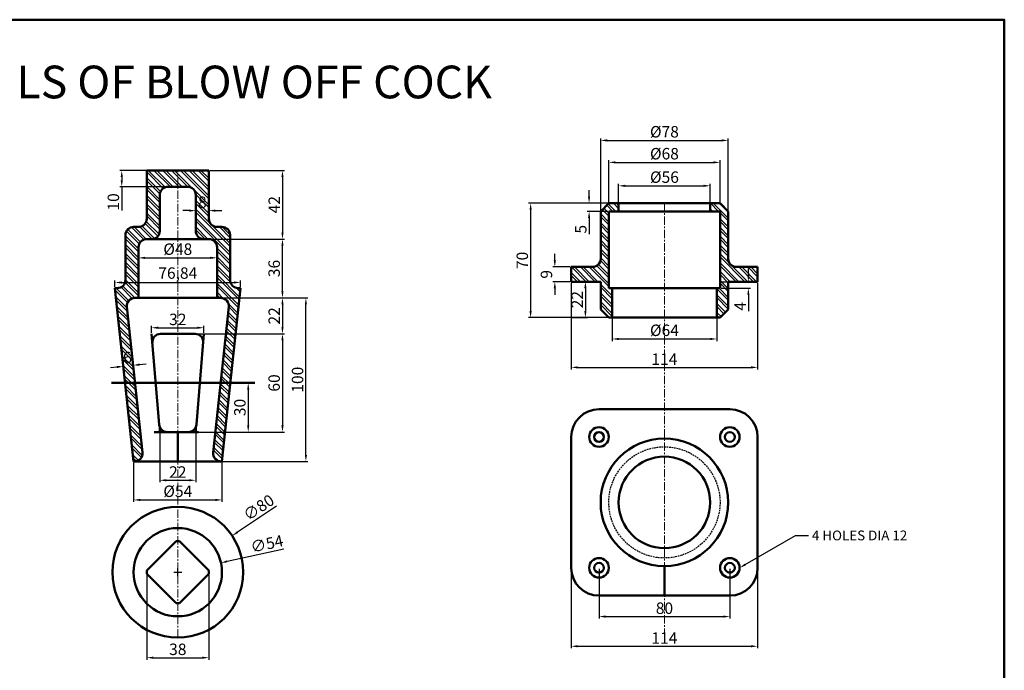
# Model space of a CAD drawing. Units: millimetres. Extents: x 49 to 1001, y -335 to 311.
# Tile 4 of 4: x 399 to 1001, y -87 to 311. Entities that reach past the tile are written whole.
import ezdxf
from ezdxf import colors
from ezdxf.entities.mleader import LeaderData, LeaderLine
from ezdxf.math import Vec2, Vec3

# ---------------------------------------------------------------- set-up
doc = ezdxf.new("R2010")
doc.units = ezdxf.units.MM
doc.header["$LTSCALE"] = 0.4
doc.linetypes.add('CENTER', pattern=[50.8, 31.75, -6.35, 6.35, -6.35])
doc.linetypes.add('HIDDEN', pattern=[9.525, 6.35, -3.175])
for name, color, linetype, lineweight in [('M-CNTR', 1, 'CENTER', 18), ('M-DIMS', 2, 'Continuous', 25), ('M-HATC', 8, 'Continuous', 18), ('M-HIDN', 6, 'HIDDEN', 25), ('M-OUTL', 7, 'Continuous', 50), ('M-TEXT', 3, 'Continuous', 25)]:
    doc.layers.add(name, color=color, linetype=linetype, lineweight=lineweight)
doc.styles.get("Standard").update_dxf_attribs({"font": 'arial.ttf'})
doc.dimstyles.new('ISO-25', dxfattribs={"dimtxt": 7, "dimasz": 4, "dimexe": 1.25, "dimexo": 0.625, "dimtad": 1, "dimtxsty": 'Standard', "dimcen": 2.5, "dimadec": 0, "dimazin": 0, "dimtfac": 1, "dimtofl": 0, "dimtmove": 0, "dimatfit": 3, "dimfxl": 1, "dimarcsym": 0})

# ---------------------------------------------------------------- blocks, each defined once
blk = doc.blocks.new('*D24')
at = {"layer": 'Defpoints', "color": 0, "ltscale": 0.4, "transparency": 16777216}
for p in [(495.83, 219.19), (461.55, 209.19), (495.83, 209.19)]:
    blk.add_point(p, dxfattribs=at)
at = {"layer": 'M-DIMS', "color": 0, "lineweight": -2, "ltscale": 0.4, "transparency": 16777216}
for p, q in [((495.21, 219.19), (460.3, 219.19)), ((461.55, 215.19), (461.55, 213.19)), ((495.21, 209.19), (460.3, 209.19)), ((461.55, 209.19), (461.55, 194.6))]:
    blk.add_line(p, q, dxfattribs=at)
at = {"layer": 'M-DIMS', "color": 0, "ltscale": 0.4, "transparency": 16777216}
for points in [[(460.89, 215.19), (462.22, 215.19), (461.55, 219.19)], [(460.89, 213.19), (462.22, 213.19), (461.55, 209.19)]]:
    blk.add_solid(points, dxfattribs=at)
at = {"layer": 'M-DIMS', "color": 0, "ltscale": 0.4, "transparency": 16777216, "insert": (457.35, 199.9), "char_height": 7, "attachment_point": 5, "rotation": 90}
blk.add_mtext('10', dxfattribs=at)
blk = doc.blocks.new('*D25')
at = {"layer": 'Defpoints', "color": 0, "ltscale": 0.4, "transparency": 16777216}
for p in [(514.83, 219.19), (495.83, 177.19), (559.86, 177.19)]:
    blk.add_point(p, dxfattribs=at)
at = {"layer": 'M-DIMS', "color": 0, "lineweight": -2, "ltscale": 0.4, "transparency": 16777216}
for p, q in [((515.46, 219.19), (561.11, 219.19)), ((559.86, 215.19), (559.86, 181.19)), ((496.46, 177.19), (561.11, 177.19))]:
    blk.add_line(p, q, dxfattribs=at)
at = {"layer": 'M-DIMS', "color": 0, "ltscale": 0.4, "transparency": 16777216}
for points in [[(559.19, 215.19), (560.52, 215.19), (559.86, 219.19)], [(559.19, 181.19), (560.52, 181.19), (559.86, 177.19)]]:
    blk.add_solid(points, dxfattribs=at)
at = {"layer": 'M-DIMS', "color": 0, "ltscale": 0.4, "transparency": 16777216, "insert": (555.72, 198.19), "char_height": 7, "attachment_point": 5, "rotation": 90}
blk.add_mtext('42', dxfattribs=at)
blk = doc.blocks.new('*D26')
at = {"layer": 'Defpoints', "color": 0, "ltscale": 0.4, "transparency": 16777216}
for p in [(506.83, 196.43), (514.83, 196.43), (514.83, 194.58)]:
    blk.add_point(p, dxfattribs=at)
at = {"layer": 'M-DIMS', "color": 0, "lineweight": -2, "ltscale": 0.4, "transparency": 16777216}
for p, q in [((502.83, 194.58), (498.83, 194.58)), ((506.83, 195.81), (506.83, 193.33)), ((514.83, 195.81), (514.83, 193.33)), ((518.83, 194.58), (522.83, 194.58))]:
    blk.add_line(p, q, dxfattribs=at)
at = {"layer": 'M-DIMS', "color": 0, "ltscale": 0.4, "transparency": 16777216}
for points in [[(502.83, 195.25), (502.83, 193.91), (506.83, 194.58)], [(518.83, 195.25), (518.83, 193.91), (514.83, 194.58)]]:
    blk.add_solid(points, dxfattribs=at)
at = {"layer": 'M-DIMS', "color": 0, "ltscale": 0.4, "transparency": 16777216, "insert": (510.83, 198.78), "char_height": 7, "attachment_point": 5}
blk.add_mtext('8', dxfattribs=at)
blk = doc.blocks.new('*D27')
at = {"layer": 'Defpoints', "color": 0, "ltscale": 0.4, "transparency": 16777216}
for p in [(468.83, 41.19), (522.83, 41.19), (522.83, 17.66)]:
    blk.add_point(p, dxfattribs=at)
at = {"layer": 'M-DIMS', "color": 0, "lineweight": -2, "ltscale": 0.4, "transparency": 16777216}
for p, q in [((468.83, 40.57), (468.83, 16.41)), ((522.83, 40.57), (522.83, 16.41)), ((472.83, 17.66), (518.83, 17.66))]:
    blk.add_line(p, q, dxfattribs=at)
at = {"layer": 'M-DIMS', "color": 0, "ltscale": 0.4, "transparency": 16777216}
for points in [[(472.83, 18.32), (472.83, 16.99), (468.83, 17.66)], [(518.83, 18.32), (518.83, 16.99), (522.83, 17.66)]]:
    blk.add_solid(points, dxfattribs=at)
at = {"layer": 'M-DIMS', "color": 0, "ltscale": 0.4, "transparency": 16777216, "insert": (495.83, 22.05), "char_height": 7, "attachment_point": 5}
blk.add_mtext('%%C54', dxfattribs=at)
blk = doc.blocks.new('*D28')
at = {"layer": 'Defpoints', "color": 0, "ltscale": 0.4, "transparency": 16777216}
for p in [(484.83, 59.19), (506.83, 59.19), (506.83, 29.68)]:
    blk.add_point(p, dxfattribs=at)
at = {"layer": 'M-DIMS', "color": 0, "lineweight": -2, "ltscale": 0.4, "transparency": 16777216}
for p, q in [((484.83, 58.57), (484.83, 28.43)), ((506.83, 58.57), (506.83, 28.43)), ((488.83, 29.68), (502.83, 29.68))]:
    blk.add_line(p, q, dxfattribs=at)
at = {"layer": 'M-DIMS', "color": 0, "ltscale": 0.4, "transparency": 16777216}
for points in [[(488.83, 30.35), (488.83, 29.01), (484.83, 29.68)], [(502.83, 30.35), (502.83, 29.01), (506.83, 29.68)]]:
    blk.add_solid(points, dxfattribs=at)
at = {"layer": 'M-DIMS', "color": 0, "ltscale": 0.4, "transparency": 16777216, "insert": (495.83, 33.82), "char_height": 7, "attachment_point": 5}
blk.add_mtext('22', dxfattribs=at)
blk = doc.blocks.new('*D29')
at = {"layer": 'Defpoints', "color": 0, "ltscale": 0.4, "transparency": 16777216}
for p in [(519.83, 165.71), (471.83, 161.25), (519.83, 161.25)]:
    blk.add_point(p, dxfattribs=at)
at = {"layer": 'M-DIMS', "color": 0, "lineweight": -2, "ltscale": 0.4, "transparency": 16777216}
for p, q in [((471.83, 161.88), (471.83, 166.96)), ((475.83, 165.71), (515.83, 165.71)), ((519.83, 161.88), (519.83, 166.96))]:
    blk.add_line(p, q, dxfattribs=at)
at = {"layer": 'M-DIMS', "color": 0, "ltscale": 0.4, "transparency": 16777216}
for points in [[(475.83, 166.38), (475.83, 165.04), (471.83, 165.71)], [(515.83, 166.38), (515.83, 165.04), (519.83, 165.71)]]:
    blk.add_solid(points, dxfattribs=at)
at = {"layer": 'M-DIMS', "color": 0, "ltscale": 0.4, "transparency": 16777216, "insert": (495.83, 170.11), "char_height": 7, "attachment_point": 5}
blk.add_mtext('%%C48', dxfattribs=at)
blk = doc.blocks.new('*D30')
at = {"layer": 'Defpoints', "color": 0, "ltscale": 0.4, "transparency": 16777216}
for p in [(534.25, 150.64), (457.41, 147.19), (534.25, 147.19)]:
    blk.add_point(p, dxfattribs=at)
at = {"layer": 'M-DIMS', "color": 0, "lineweight": -2, "ltscale": 0.4, "transparency": 16777216}
for p, q in [((457.41, 147.82), (457.41, 151.89)), ((461.41, 150.64), (530.25, 150.64)), ((534.25, 147.82), (534.25, 151.89))]:
    blk.add_line(p, q, dxfattribs=at)
at = {"layer": 'M-DIMS', "color": 0, "ltscale": 0.4, "transparency": 16777216}
for points in [[(461.41, 151.31), (461.41, 149.98), (457.41, 150.64)], [(530.25, 151.31), (530.25, 149.98), (534.25, 150.64)]]:
    blk.add_solid(points, dxfattribs=at)
at = {"layer": 'M-DIMS', "color": 0, "ltscale": 0.4, "transparency": 16777216, "insert": (495.83, 155.48), "char_height": 7, "attachment_point": 5}
blk.add_mtext('76,84', dxfattribs=at)
blk = doc.blocks.new('*D31')
at = {"layer": 'Defpoints', "color": 0, "ltscale": 0.4, "transparency": 16777216}
for p in [(505.76, 177.19), (559.86, 177.19), (512.69, 141.19)]:
    blk.add_point(p, dxfattribs=at)
at = {"layer": 'M-DIMS', "color": 0, "lineweight": -2, "ltscale": 0.4, "transparency": 16777216}
for p, q in [((506.39, 177.19), (561.11, 177.19)), ((559.86, 145.19), (559.86, 173.19)), ((513.32, 141.19), (561.11, 141.19))]:
    blk.add_line(p, q, dxfattribs=at)
at = {"layer": 'M-DIMS', "color": 0, "ltscale": 0.4, "transparency": 16777216}
for points in [[(559.19, 173.19), (560.52, 173.19), (559.86, 177.19)], [(559.19, 145.19), (560.52, 145.19), (559.86, 141.19)]]:
    blk.add_solid(points, dxfattribs=at)
at = {"layer": 'M-DIMS', "color": 0, "ltscale": 0.4, "transparency": 16777216, "insert": (555.66, 159.19), "char_height": 7, "attachment_point": 5, "rotation": 90}
blk.add_mtext('36', dxfattribs=at)
blk = doc.blocks.new('*D32')
at = {"layer": 'Defpoints', "color": 0, "ltscale": 0.4, "transparency": 16777216}
for p in [(505.39, 141.19), (505.39, 119.19), (559.86, 119.19)]:
    blk.add_point(p, dxfattribs=at)
at = {"layer": 'M-DIMS', "color": 0, "lineweight": -2, "ltscale": 0.4, "transparency": 16777216}
for p, q in [((506.01, 141.19), (561.11, 141.19)), ((559.86, 137.19), (559.86, 123.19)), ((506.01, 119.19), (561.11, 119.19))]:
    blk.add_line(p, q, dxfattribs=at)
at = {"layer": 'M-DIMS', "color": 0, "ltscale": 0.4, "transparency": 16777216}
for points in [[(559.19, 137.19), (560.52, 137.19), (559.86, 141.19)], [(559.19, 123.19), (560.52, 123.19), (559.86, 119.19)]]:
    blk.add_solid(points, dxfattribs=at)
at = {"layer": 'M-DIMS', "color": 0, "ltscale": 0.4, "transparency": 16777216, "insert": (555.72, 130.19), "char_height": 7, "attachment_point": 5, "rotation": 90}
blk.add_mtext('22', dxfattribs=at)
blk = doc.blocks.new('*D33')
at = {"layer": 'Defpoints', "color": 0, "ltscale": 0.4, "transparency": 16777216}
for p in [(495.83, 119.19), (495.83, 59.19), (559.86, 59.19)]:
    blk.add_point(p, dxfattribs=at)
at = {"layer": 'M-DIMS', "color": 0, "lineweight": -2, "ltscale": 0.4, "transparency": 16777216}
for p, q in [((496.46, 119.19), (561.11, 119.19)), ((559.86, 115.19), (559.86, 63.19)), ((496.46, 59.19), (561.11, 59.19))]:
    blk.add_line(p, q, dxfattribs=at)
at = {"layer": 'M-DIMS', "color": 0, "ltscale": 0.4, "transparency": 16777216}
for points in [[(559.19, 115.19), (560.52, 115.19), (559.86, 119.19)], [(559.19, 63.19), (560.52, 63.19), (559.86, 59.19)]]:
    blk.add_solid(points, dxfattribs=at)
at = {"layer": 'M-DIMS', "color": 0, "ltscale": 0.4, "transparency": 16777216, "insert": (555.66, 89.19), "char_height": 7, "attachment_point": 5, "rotation": 90}
blk.add_mtext('60', dxfattribs=at)
blk = doc.blocks.new('*D34')
at = {"layer": 'Defpoints', "color": 0, "ltscale": 0.4, "transparency": 16777216}
for p in [(495.83, 141.19), (574.18, 141.19), (495.83, 41.19)]:
    blk.add_point(p, dxfattribs=at)
at = {"layer": 'M-DIMS', "color": 0, "lineweight": -2, "ltscale": 0.4, "transparency": 16777216}
for p, q in [((496.46, 141.19), (575.43, 141.19)), ((574.18, 45.19), (574.18, 137.19)), ((496.46, 41.19), (575.43, 41.19))]:
    blk.add_line(p, q, dxfattribs=at)
at = {"layer": 'M-DIMS', "color": 0, "ltscale": 0.4, "transparency": 16777216}
for points in [[(573.52, 137.19), (574.85, 137.19), (574.18, 141.19)], [(573.52, 45.19), (574.85, 45.19), (574.18, 41.19)]]:
    blk.add_solid(points, dxfattribs=at)
at = {"layer": 'M-DIMS', "color": 0, "ltscale": 0.4, "transparency": 16777216, "insert": (569.98, 91.19), "char_height": 7, "attachment_point": 5, "rotation": 90}
blk.add_mtext('100', dxfattribs=at)
blk = doc.blocks.new('*D35')
at = {"layer": 'Defpoints', "color": 0, "ltscale": 0.4, "transparency": 16777216}
for p in [(535.16, 89.19), (535.16, 59.19), (538.91, 59.19)]:
    blk.add_point(p, dxfattribs=at)
at = {"layer": 'M-DIMS', "color": 0, "lineweight": -2, "ltscale": 0.4, "transparency": 16777216}
for p, q in [((535.79, 89.19), (540.16, 89.19)), ((538.91, 85.19), (538.91, 63.19)), ((535.79, 59.19), (540.16, 59.19))]:
    blk.add_line(p, q, dxfattribs=at)
at = {"layer": 'M-DIMS', "color": 0, "ltscale": 0.4, "transparency": 16777216}
for points in [[(538.24, 85.19), (539.58, 85.19), (538.91, 89.19)], [(538.24, 63.19), (539.58, 63.19), (538.91, 59.19)]]:
    blk.add_solid(points, dxfattribs=at)
at = {"layer": 'M-DIMS', "color": 0, "ltscale": 0.4, "transparency": 16777216, "insert": (534.71, 74.19), "char_height": 7, "attachment_point": 5, "rotation": 90}
blk.add_mtext('30', dxfattribs=at)
blk = doc.blocks.new('*D36')
at = {"layer": 'Defpoints', "color": 0, "ltscale": 0.4, "transparency": 16777216}
for p in [(511.83, 122.96), (479.83, 119.19), (511.83, 119.19)]:
    blk.add_point(p, dxfattribs=at)
at = {"layer": 'M-DIMS', "color": 0, "lineweight": -2, "ltscale": 0.4, "transparency": 16777216}
for p, q in [((479.83, 119.82), (479.83, 124.21)), ((483.83, 122.96), (507.83, 122.96)), ((511.83, 119.82), (511.83, 124.21))]:
    blk.add_line(p, q, dxfattribs=at)
at = {"layer": 'M-DIMS', "color": 0, "ltscale": 0.4, "transparency": 16777216}
for points in [[(483.83, 123.62), (483.83, 122.29), (479.83, 122.96)], [(507.83, 123.62), (507.83, 122.29), (511.83, 122.96)]]:
    blk.add_solid(points, dxfattribs=at)
at = {"layer": 'M-DIMS', "color": 0, "ltscale": 0.4, "transparency": 16777216, "insert": (495.83, 127.16), "char_height": 7, "attachment_point": 5}
blk.add_mtext('32', dxfattribs=at)
blk = doc.blocks.new('*D37')
at = {"layer": 'Defpoints', "color": 0, "ltscale": 0.4, "transparency": 16777216}
for p in [(468.53, 99.98), (463.12, 94.19), (469.09, 94.84)]:
    blk.add_point(p, dxfattribs=at)
at = {"layer": 'M-DIMS', "color": 0, "lineweight": -2, "ltscale": 0.4, "transparency": 16777216}
for p, q in [((458.59, 98.91), (454.62, 98.48)), ((463.06, 94.81), (462.44, 100.58)), ((469.02, 95.46), (468.4, 101.23)), ((472.51, 100.41), (476.49, 100.84))]:
    blk.add_line(p, q, dxfattribs=at)
at = {"layer": 'M-DIMS', "color": 0, "ltscale": 0.4, "transparency": 16777216}
for points in [[(458.52, 99.58), (458.66, 98.25), (462.57, 99.34)], [(472.44, 101.08), (472.58, 99.75), (468.53, 99.98)]]:
    blk.add_solid(points, dxfattribs=at)
at = {"layer": 'M-DIMS', "color": 0, "ltscale": 0.4, "transparency": 16777216, "insert": (465.1, 103.84), "char_height": 7, "attachment_point": 5, "rotation": 6.14894}
blk.add_mtext('6', dxfattribs=at)
blk = doc.blocks.new('*D38')
at = {"layer": 'Defpoints', "color": 0, "ltscale": 0.4, "transparency": 16777216}
for p in [(476.83, -27.52), (514.83, -27.52), (514.83, -78.82)]:
    blk.add_point(p, dxfattribs=at)
at = {"layer": 'M-DIMS', "color": 0, "lineweight": -2, "ltscale": 0.4, "transparency": 16777216}
for p, q in [((476.83, -28.15), (476.83, -80.07)), ((514.83, -28.15), (514.83, -80.07)), ((480.83, -78.82), (510.83, -78.82))]:
    blk.add_line(p, q, dxfattribs=at)
at = {"layer": 'M-DIMS', "color": 0, "ltscale": 0.4, "transparency": 16777216}
for points in [[(480.83, -78.15), (480.83, -79.48), (476.83, -78.82)], [(510.83, -78.15), (510.83, -79.48), (514.83, -78.82)]]:
    blk.add_solid(points, dxfattribs=at)
at = {"layer": 'M-DIMS', "color": 0, "ltscale": 0.4, "transparency": 16777216, "insert": (495.83, -74.61), "char_height": 7, "attachment_point": 5}
blk.add_mtext('38', dxfattribs=at)
blk = doc.blocks.new('*D39')
at = {"layer": 'Defpoints', "color": 0, "ltscale": 0.4, "transparency": 16777216}
for p in [(529.06, -4.25), (462.61, -48.79)]:
    blk.add_point(p, dxfattribs=at)
at = {"layer": 'M-DIMS', "color": 0, "lineweight": -2, "ltscale": 0.4, "transparency": 16777216}
for p, q in [((556.12, 13.88), (532.38, -2.03)), ((495.83, -29.02), (495.83, -24.02)), ((493.33, -26.52), (498.33, -26.52))]:
    blk.add_line(p, q, dxfattribs=at)
at = {"layer": 'M-DIMS', "color": 0, "ltscale": 0.4, "transparency": 16777216}
blk.add_solid([(532.01, -1.47), (532.76, -2.58), (529.06, -4.25)], dxfattribs=at)
at = {"layer": 'M-DIMS', "color": 0, "ltscale": 0.4, "transparency": 16777216, "insert": (545.83, 12.28), "char_height": 7, "attachment_point": 5, "rotation": 33.82924}
blk.add_mtext('∅80', dxfattribs=at)
blk = doc.blocks.new('*D40')
at = {"layer": 'Defpoints', "color": 0, "ltscale": 0.4, "transparency": 16777216}
for p in [(522.21, -20.76), (469.46, -32.29)]:
    blk.add_point(p, dxfattribs=at)
at = {"layer": 'M-DIMS', "color": 0, "lineweight": -2, "ltscale": 0.4, "transparency": 16777216}
for p, q in [((560.68, -12.35), (526.12, -19.9)), ((495.83, -29.02), (495.83, -24.02)), ((493.33, -26.52), (498.33, -26.52))]:
    blk.add_line(p, q, dxfattribs=at)
at = {"layer": 'M-DIMS', "color": 0, "ltscale": 0.4, "transparency": 16777216}
blk.add_solid([(525.98, -19.25), (526.26, -20.55), (522.21, -20.76)], dxfattribs=at)
at = {"layer": 'M-DIMS', "color": 0, "ltscale": 0.4, "transparency": 16777216, "insert": (550.53, -10.07), "char_height": 7, "attachment_point": 5, "rotation": 12.32808}
blk.add_mtext('∅54', dxfattribs=at)
blk = doc.blocks.new('*D41')
at = {"layer": 'Defpoints', "color": 0, "ltscale": 0.4, "transparency": 16777216}
for p in [(832.47, 237.52), (754.47, 194.13), (832.47, 194.13)]:
    blk.add_point(p, dxfattribs=at)
at = {"layer": 'M-DIMS', "color": 0, "lineweight": -2, "ltscale": 0.4, "transparency": 16777216}
for p, q in [((754.47, 194.76), (754.47, 238.77)), ((758.47, 237.52), (828.47, 237.52)), ((832.47, 194.76), (832.47, 238.77))]:
    blk.add_line(p, q, dxfattribs=at)
at = {"layer": 'M-DIMS', "color": 0, "ltscale": 0.4, "transparency": 16777216}
for points in [[(758.47, 238.19), (758.47, 236.85), (754.47, 237.52)], [(828.47, 238.19), (828.47, 236.85), (832.47, 237.52)]]:
    blk.add_solid(points, dxfattribs=at)
at = {"layer": 'M-DIMS', "color": 0, "ltscale": 0.4, "transparency": 16777216, "insert": (793.47, 241.92), "char_height": 7, "attachment_point": 5}
blk.add_mtext('%%C78', dxfattribs=at)
blk = doc.blocks.new('*D42')
at = {"layer": 'Defpoints', "color": 0, "ltscale": 0.4, "transparency": 16777216}
for p in [(821.47, 209.76), (765.47, 199.13), (821.47, 199.13)]:
    blk.add_point(p, dxfattribs=at)
at = {"layer": 'M-DIMS', "color": 0, "lineweight": -2, "ltscale": 0.4, "transparency": 16777216}
for p, q in [((765.47, 199.76), (765.47, 211.01)), ((821.47, 199.76), (821.47, 211.01)), ((769.47, 209.76), (817.47, 209.76))]:
    blk.add_line(p, q, dxfattribs=at)
at = {"layer": 'M-DIMS', "color": 0, "ltscale": 0.4, "transparency": 16777216}
for points in [[(769.47, 210.42), (769.47, 209.09), (765.47, 209.76)], [(817.47, 210.42), (817.47, 209.09), (821.47, 209.76)]]:
    blk.add_solid(points, dxfattribs=at)
at = {"layer": 'M-DIMS', "color": 0, "ltscale": 0.4, "transparency": 16777216, "insert": (793.47, 214.15), "char_height": 7, "attachment_point": 5}
blk.add_mtext('%%C56', dxfattribs=at)
blk = doc.blocks.new('*D43')
at = {"layer": 'Defpoints', "color": 0, "ltscale": 0.4, "transparency": 16777216}
for p in [(827.47, 224.09), (759.47, 199.13), (827.47, 199.13)]:
    blk.add_point(p, dxfattribs=at)
at = {"layer": 'M-DIMS', "color": 0, "lineweight": -2, "ltscale": 0.4, "transparency": 16777216}
for p, q in [((759.47, 199.76), (759.47, 225.34)), ((763.47, 224.09), (823.47, 224.09)), ((827.47, 199.76), (827.47, 225.34))]:
    blk.add_line(p, q, dxfattribs=at)
at = {"layer": 'M-DIMS', "color": 0, "ltscale": 0.4, "transparency": 16777216}
for points in [[(763.47, 224.76), (763.47, 223.43), (759.47, 224.09)], [(823.47, 224.76), (823.47, 223.43), (827.47, 224.09)]]:
    blk.add_solid(points, dxfattribs=at)
at = {"layer": 'M-DIMS', "color": 0, "ltscale": 0.4, "transparency": 16777216, "insert": (793.47, 228.49), "char_height": 7, "attachment_point": 5}
blk.add_mtext('%%C68', dxfattribs=at)
blk = doc.blocks.new('*D44')
at = {"layer": 'Defpoints', "color": 0, "ltscale": 0.4, "transparency": 16777216}
for p in [(759.47, 199.13), (747.39, 194.13), (759.47, 194.13)]:
    blk.add_point(p, dxfattribs=at)
at = {"layer": 'M-DIMS', "color": 0, "lineweight": -2, "ltscale": 0.4, "transparency": 16777216}
for p, q in [((747.39, 203.13), (747.39, 207.13)), ((758.84, 199.13), (746.14, 199.13)), ((758.84, 194.13), (746.14, 194.13)), ((747.39, 190.13), (747.39, 180.24))]:
    blk.add_line(p, q, dxfattribs=at)
at = {"layer": 'M-DIMS', "color": 0, "ltscale": 0.4, "transparency": 16777216}
for points in [[(746.72, 203.13), (748.05, 203.13), (747.39, 199.13)], [(746.72, 190.13), (748.05, 190.13), (747.39, 194.13)]]:
    blk.add_solid(points, dxfattribs=at)
at = {"layer": 'M-DIMS', "color": 0, "ltscale": 0.4, "transparency": 16777216, "insert": (743.2, 183.19), "char_height": 7, "attachment_point": 5, "rotation": 90}
blk.add_mtext('5', dxfattribs=at)
blk = doc.blocks.new('*D45')
at = {"layer": 'Defpoints', "color": 0, "ltscale": 0.4, "transparency": 16777216}
for p in [(777.9, 199.13), (711.63, 129.13), (777.9, 129.13)]:
    blk.add_point(p, dxfattribs=at)
at = {"layer": 'M-DIMS', "color": 0, "lineweight": -2, "ltscale": 0.4, "transparency": 16777216}
for p, q in [((777.28, 199.13), (710.38, 199.13)), ((711.63, 195.13), (711.63, 133.13)), ((777.28, 129.13), (710.38, 129.13))]:
    blk.add_line(p, q, dxfattribs=at)
at = {"layer": 'M-DIMS', "color": 0, "ltscale": 0.4, "transparency": 16777216}
for points in [[(710.96, 195.13), (712.29, 195.13), (711.63, 199.13)], [(710.96, 133.13), (712.29, 133.13), (711.63, 129.13)]]:
    blk.add_solid(points, dxfattribs=at)
at = {"layer": 'M-DIMS', "color": 0, "ltscale": 0.4, "transparency": 16777216, "insert": (707.43, 164.13), "char_height": 7, "attachment_point": 5, "rotation": 90}
blk.add_mtext('70', dxfattribs=at)
blk = doc.blocks.new('*D46')
at = {"layer": 'Defpoints', "color": 0, "ltscale": 0.4, "transparency": 16777216}
for p in [(736.47, 160.13), (726.42, 151.13), (736.47, 151.13)]:
    blk.add_point(p, dxfattribs=at)
at = {"layer": 'M-DIMS', "color": 0, "lineweight": -2, "ltscale": 0.4, "transparency": 16777216}
for p, q in [((726.42, 164.13), (726.42, 168.13)), ((735.84, 160.13), (725.17, 160.13)), ((735.84, 151.13), (725.17, 151.13)), ((726.42, 147.13), (726.42, 143.13))]:
    blk.add_line(p, q, dxfattribs=at)
at = {"layer": 'M-DIMS', "color": 0, "ltscale": 0.4, "transparency": 16777216}
for points in [[(725.76, 164.13), (727.09, 164.13), (726.42, 160.13)], [(725.76, 147.13), (727.09, 147.13), (726.42, 151.13)]]:
    blk.add_solid(points, dxfattribs=at)
at = {"layer": 'M-DIMS', "color": 0, "ltscale": 0.4, "transparency": 16777216, "insert": (722.22, 155.63), "char_height": 7, "attachment_point": 5, "rotation": 90}
blk.add_mtext('9', dxfattribs=at)
blk = doc.blocks.new('*D47')
at = {"layer": 'Defpoints', "color": 0, "ltscale": 0.4, "transparency": 16777216}
for p in [(736.47, 151.13), (736.47, 129.13), (745.12, 129.13)]:
    blk.add_point(p, dxfattribs=at)
at = {"layer": 'M-DIMS', "color": 0, "lineweight": -2, "ltscale": 0.4, "transparency": 16777216}
for p, q in [((737.09, 151.13), (746.37, 151.13)), ((745.12, 147.13), (745.12, 133.13)), ((737.09, 129.13), (746.37, 129.13))]:
    blk.add_line(p, q, dxfattribs=at)
at = {"layer": 'M-DIMS', "color": 0, "ltscale": 0.4, "transparency": 16777216}
for points in [[(744.46, 147.13), (745.79, 147.13), (745.12, 151.13)], [(744.46, 133.13), (745.79, 133.13), (745.12, 129.13)]]:
    blk.add_solid(points, dxfattribs=at)
at = {"layer": 'M-DIMS', "color": 0, "ltscale": 0.4, "transparency": 16777216, "insert": (740.98, 140.13), "char_height": 7, "attachment_point": 5, "rotation": 90}
blk.add_mtext('22', dxfattribs=at)
blk = doc.blocks.new('*D48')
at = {"layer": 'Defpoints', "color": 0, "ltscale": 0.4, "transparency": 16777216}
for p in [(827.47, 151.13), (827.47, 147.13), (844.79, 147.13)]:
    blk.add_point(p, dxfattribs=at)
at = {"layer": 'M-DIMS', "color": 0, "lineweight": -2, "ltscale": 0.4, "transparency": 16777216}
for p, q in [((844.79, 155.13), (844.79, 159.13)), ((828.09, 151.13), (846.04, 151.13)), ((828.09, 147.13), (846.04, 147.13)), ((844.79, 143.13), (844.79, 133.04))]:
    blk.add_line(p, q, dxfattribs=at)
at = {"layer": 'M-DIMS', "color": 0, "ltscale": 0.4, "transparency": 16777216}
for points in [[(844.12, 155.13), (845.45, 155.13), (844.79, 151.13)], [(844.12, 143.13), (845.45, 143.13), (844.79, 147.13)]]:
    blk.add_solid(points, dxfattribs=at)
at = {"layer": 'M-DIMS', "color": 0, "ltscale": 0.4, "transparency": 16777216, "insert": (840.66, 136.09), "char_height": 7, "attachment_point": 5, "rotation": 90}
blk.add_mtext('4', dxfattribs=at)
blk = doc.blocks.new('*D49')
at = {"layer": 'Defpoints', "color": 0, "ltscale": 0.4, "transparency": 16777216}
for p in [(761.47, 129.13), (825.47, 129.13), (825.47, 116.1)]:
    blk.add_point(p, dxfattribs=at)
at = {"layer": 'M-DIMS', "color": 0, "lineweight": -2, "ltscale": 0.4, "transparency": 16777216}
for p, q in [((761.47, 128.51), (761.47, 114.85)), ((825.47, 128.51), (825.47, 114.85)), ((765.47, 116.1), (821.47, 116.1))]:
    blk.add_line(p, q, dxfattribs=at)
at = {"layer": 'M-DIMS', "color": 0, "ltscale": 0.4, "transparency": 16777216}
for points in [[(765.47, 116.77), (765.47, 115.43), (761.47, 116.1)], [(821.47, 116.77), (821.47, 115.43), (825.47, 116.1)]]:
    blk.add_solid(points, dxfattribs=at)
at = {"layer": 'M-DIMS', "color": 0, "ltscale": 0.4, "transparency": 16777216, "insert": (793.47, 120.49), "char_height": 7, "attachment_point": 5}
blk.add_mtext('%%C64', dxfattribs=at)
blk = doc.blocks.new('*D50')
at = {"layer": 'Defpoints', "color": 0, "ltscale": 0.4, "transparency": 16777216}
for p in [(736.47, 151.13), (850.47, 151.13), (850.47, 98.71)]:
    blk.add_point(p, dxfattribs=at)
at = {"layer": 'M-DIMS', "color": 0, "lineweight": -2, "ltscale": 0.4, "transparency": 16777216}
for p, q in [((736.47, 150.51), (736.47, 97.46)), ((850.47, 150.51), (850.47, 97.46)), ((740.47, 98.71), (846.47, 98.71))]:
    blk.add_line(p, q, dxfattribs=at)
at = {"layer": 'M-DIMS', "color": 0, "ltscale": 0.4, "transparency": 16777216}
for points in [[(740.47, 99.38), (740.47, 98.05), (736.47, 98.71)], [(846.47, 99.38), (846.47, 98.05), (850.47, 98.71)]]:
    blk.add_solid(points, dxfattribs=at)
at = {"layer": 'M-DIMS', "color": 0, "ltscale": 0.4, "transparency": 16777216, "insert": (793.47, 102.85), "char_height": 7, "attachment_point": 5}
blk.add_mtext('114', dxfattribs=at)
blk = doc.blocks.new('*D51')
at = {"layer": 'Defpoints', "color": 0, "ltscale": 0.4, "transparency": 16777216}
for p in [(753.47, -23.85), (833.47, -23.85), (833.47, -53.67)]:
    blk.add_point(p, dxfattribs=at)
at = {"layer": 'M-DIMS', "color": 0, "lineweight": -2, "ltscale": 0.4, "transparency": 16777216}
for p, q in [((753.47, -24.48), (753.47, -54.92)), ((833.47, -24.48), (833.47, -54.92)), ((757.47, -53.67), (829.47, -53.67))]:
    blk.add_line(p, q, dxfattribs=at)
at = {"layer": 'M-DIMS', "color": 0, "ltscale": 0.4, "transparency": 16777216}
for points in [[(757.47, -53), (757.47, -54.34), (753.47, -53.67)], [(829.47, -53), (829.47, -54.34), (833.47, -53.67)]]:
    blk.add_solid(points, dxfattribs=at)
at = {"layer": 'M-DIMS', "color": 0, "ltscale": 0.4, "transparency": 16777216, "insert": (793.47, -49.47), "char_height": 7, "attachment_point": 5}
blk.add_mtext('80', dxfattribs=at)
blk = doc.blocks.new('*D52')
at = {"layer": 'Defpoints', "color": 0, "ltscale": 0.4, "transparency": 16777216}
for p in [(736.47, -9.14), (850.47, -9.14), (850.47, -71.82)]:
    blk.add_point(p, dxfattribs=at)
at = {"layer": 'M-DIMS', "color": 0, "lineweight": -2, "ltscale": 0.4, "transparency": 16777216}
for p, q in [((736.47, -9.76), (736.47, -73.07)), ((850.47, -9.76), (850.47, -73.07)), ((740.47, -71.82), (846.47, -71.82))]:
    blk.add_line(p, q, dxfattribs=at)
at = {"layer": 'M-DIMS', "color": 0, "ltscale": 0.4, "transparency": 16777216}
for points in [[(740.47, -71.15), (740.47, -72.48), (736.47, -71.82)], [(846.47, -71.15), (846.47, -72.48), (850.47, -71.82)]]:
    blk.add_solid(points, dxfattribs=at)
at = {"layer": 'M-DIMS', "color": 0, "ltscale": 0.4, "transparency": 16777216, "insert": (793.47, -67.68), "char_height": 7, "attachment_point": 5}
blk.add_mtext('114', dxfattribs=at)
blk = doc.blocks.new('BOLT-HOLE-12')
at = {"ltscale": 0.4}
for radius in [6, 3]:
    blk.add_circle((6, 6), radius, dxfattribs=at)

msp = doc.modelspace()

# ---------------------------------------------------------------- hatches: boundary and pattern name
at = {"layer": 'M-HATC', "ltscale": 0.4}
h = msp.add_hatch(dxfattribs=at)
h.set_pattern_fill('ANSI32', color=256, scale=0.4, angle=90)
h.paths.add_polyline_path([(468.8337, 41.1927), (469.3008, 41.1927, 0.44600763), (474.272, 46.7282), (464.6914, 135.6571, -0.44600763), (469.6627, 141.1927), (471.8337, 141.1927), (471.8337, 172.1927, -0.41421356), (476.8337, 177.1927), (479.8337, 177.1927, 0.41421356), (484.8337, 182.1927), (484.8337, 204.1927, -0.41421356), (489.8337, 209.1927), (495.8337, 209.1927), (495.8337, 219.1927), (476.8337, 219.1927), (476.8337, 189.6089, -0.41421356), (471.8337, 184.6089), (468.8337, 184.6089, 0.41421356), (463.8337, 179.6089), (463.8337, 152.1927, -0.41421356), (458.8337, 147.1927), (457.414, 147.1927)])
h.paths.add_polyline_path([(517.3953, 46.7282, 0.44600763), (522.3666, 41.1927), (522.8337, 41.1927), (534.2534, 147.1927), (532.8337, 147.1927, -0.41421356), (527.8337, 152.1927), (527.8337, 179.6089, 0.41421356), (522.8337, 184.6089), (519.8337, 184.6089, -0.41421356), (514.8337, 189.6089), (514.8337, 219.1927), (495.8337, 219.1927), (495.8337, 209.1927), (501.8337, 209.1927, -0.41421356), (506.8337, 204.1927), (506.8337, 182.1927, 0.41421356), (511.8337, 177.1927), (514.8337, 177.1927, -0.41421356), (519.8337, 172.1927), (519.8337, 141.1927), (522.0047, 141.1927, -0.44600763), (526.9759, 135.6571)])
h = msp.add_hatch(dxfattribs=at)
h.set_pattern_fill('ANSI32', color=256, scale=0.4, angle=90)
h.set_pattern_definition([(135, (-124.905, -72.114), (-2.694077, -2.694077), []), (135, (-124.905, -70.318), (-2.694077, -2.694077), [])])
h.paths.add_polyline_path([(759.4668, 194.134), (765.4668, 194.134), (765.4668, 199.134), (759.4668, 199.134), (754.4668, 194.134), (754.4668, 165.134, -0.41421356), (749.4668, 160.134), (736.4668, 160.134), (736.4668, 151.134), (754.4668, 151.134), (754.4668, 134.134), (759.4668, 129.134), (761.4668, 129.134), (761.4668, 147.134), (759.4668, 147.134)])
h.paths.add_polyline_path([(832.4668, 151.134), (850.4668, 151.134), (850.4668, 160.134), (837.4668, 160.134, -0.41421356), (832.4668, 165.134), (832.4668, 194.134), (827.4668, 199.134), (821.4668, 199.134), (821.4668, 194.134), (827.4668, 194.134), (827.4668, 147.134), (825.4668, 147.134), (825.4668, 129.134), (827.4668, 129.134), (832.4668, 134.134)])

# ---------------------------------------------------------------- linework, layer by layer
at = {"layer": 'M-CNTR', "ltscale": 0.4}
for p, q in [((495.8337, -66.4047), (495.8337, 219.1927)), ((793.4668, 199.134), (793.4668, -69.9009))]:
    msp.add_line(p, q, dxfattribs=at)
at = {"layer": 'M-HIDN', "ltscale": 0.4}
msp.add_circle((793.4668, 16.1491), 34, dxfattribs=at)
at = {"layer": 'M-OUTL', "ltscale": 0.4}
for p, q in [((476.8337, 219.1927), (514.8337, 219.1927)), ((476.8337, 189.6089), (476.8337, 219.1927)), ((514.8337, 219.1927), (514.8337, 189.6089)), ((759.4668, 199.134), (754.4668, 194.134)), ((759.4668, 199.134), (827.4668, 199.134)), ((765.4668, 199.134), (765.4668, 194.134)), ((821.4668, 199.134), (821.4668, 194.134)), ((827.4668, 199.134), (832.4668, 194.134)), ((754.4668, 165.134), (754.4668, 194.134)), ((759.4668, 194.134), (827.4668, 194.134)), ((759.4668, 194.134), (759.4668, 147.134)), ((827.4668, 194.134), (827.4668, 147.134)), ((832.4668, 194.134), (832.4668, 165.134)), ((471.8337, 184.6089), (468.8337, 184.6089)), ((519.8337, 184.6089), (522.8337, 184.6089)), ((463.8337, 152.1927), (463.8337, 179.6089)), ((476.8337, 177.1927), (479.8337, 177.1927)), ((478.3337, 177.1927), (511.8337, 177.1927)), ((511.8337, 177.1927), (514.8337, 177.1927)), ((527.8337, 152.1927), (527.8337, 179.6089)), ((736.4668, 160.134), (736.4668, 151.134)), ((749.4668, 160.134), (736.4668, 160.134)), ((850.4668, 160.134), (837.4668, 160.134)), ((850.4668, 160.134), (850.4668, 151.134)), ((754.4668, 151.134), (736.4668, 151.134)), ((754.4668, 134.134), (754.4668, 151.134)), ((850.4668, 151.134), (832.4668, 151.134)), ((832.4668, 151.134), (832.4668, 134.134)), ((468.8337, 41.1927), (457.414, 147.1927)), ((457.414, 147.1927), (458.8337, 147.1927)), ((522.8337, 41.1927), (534.2534, 147.1927)), ((532.8337, 147.1927), (534.2534, 147.1927)), ((827.4668, 147.134), (759.4668, 147.134)), ((761.4668, 147.134), (761.4668, 129.134)), ((825.4668, 147.134), (825.4668, 129.134)), ((469.6627, 141.1927), (471.8337, 141.1927)), ((471.8337, 141.1927), (519.8337, 141.1927)), ((519.8337, 141.1927), (522.0047, 141.1927)), ((474.272, 46.7282), (464.6914, 135.6571)), ((517.3953, 46.7282), (526.9759, 135.6571)), ((754.4668, 134.134), (759.4668, 129.134)), ((832.4668, 134.134), (827.4668, 129.134)), ((827.4668, 129.134), (759.4668, 129.134)), ((484.4516, 63.7774), (479.8337, 119.1927)), ((495.8337, 119.1927), (485.2677, 119.1927)), ((495.8337, 119.1927), (506.3997, 119.1927)), ((507.2157, 63.7774), (511.8337, 119.1927)), ((543.0434, 89.1927), (455.2612, 89.1927)), ((484.8337, 62.2346), (484.8337, 59.1927)), ((506.8337, 62.2346), (506.8337, 59.1927)), ((495.8337, 59.1927), (481.4154, 59.1927)), ((495.8337, 59.1927), (508.556, 59.1927)), ((495.8337, 59.1927), (495.8337, 41.1927)), ((468.8337, 41.1927), (469.3008, 41.1927)), ((522.8337, 41.1927), (468.8337, 41.1927)), ((522.3666, 41.1927), (522.8337, 41.1927)), ((494.8337, -7.522), (496.8337, -7.522)), ((793.4668, -40.8509), (793.4668, -22.8509)), ((476.8337, -27.522), (476.8337, -25.522)), ((514.8337, -27.522), (514.8337, -25.522)), ((494.8337, -45.522), (496.8337, -45.522))]:
    msp.add_line(p, q, dxfattribs=at)
msp.add_lwpolyline([(48.6466, 311.3462), (1001.3348, 311.3462), (1001.3348, -335.0483), (48.6466, -335.0483)], close=True, dxfattribs=at)
for points in [[(479.8337, 177.1927, 0.41421356), (484.8337, 182.1927), (484.8337, 204.1927, -0.41421356), (489.8337, 209.1927), (501.8337, 209.1927, -0.41421356), (506.8337, 204.1927), (506.8337, 182.1927, 0.41421356), (511.8337, 177.1927)], [(471.8337, 141.1927), (471.8337, 172.1927, -0.41421356), (476.8337, 177.1927)], [(519.8337, 141.1927), (519.8337, 172.1927, 0.41421356), (514.8337, 177.1927)]]:
    msp.add_lwpolyline(points, format="xyb", dxfattribs=at)
msp.add_lwpolyline([(753.4668, 73.1491), (833.4668, 73.1491, -0.41421356), (850.4668, 56.1491), (850.4668, -23.8509, -0.41421356), (833.4668, -40.8509), (753.4668, -40.8509, -0.41421356), (736.4668, -23.8509), (736.4668, 56.1491, -0.41421356)], format="xyb", close=True, dxfattribs=at)
for points in [[(494.8337, -7.522), (476.8337, -25.522)], [(514.8337, -25.522), (496.8337, -7.522)], [(476.8337, -27.522), (494.8337, -45.522)], [(496.8337, -45.522), (514.8337, -27.522)]]:
    msp.add_lwpolyline(points, dxfattribs=at)
for centre, radius in [((793.4668, 16.1491), 39), ((793.4668, 16.1491), 28), ((495.8337, -26.522), 40), ((495.8337, -26.522), 27)]:
    msp.add_circle(centre, radius, dxfattribs=at)
for centre, start, end in [((471.8337, 189.6089), 270, 0), ((519.8337, 189.6089), 180, 270), ((468.8337, 179.6089), 90, 180), ((522.8337, 179.6089), 360, 90), ((749.4668, 165.134), 270, 0), ((837.4668, 165.134), 180, 270), ((458.8337, 152.1927), 270, 360), ((532.8337, 152.1927), 180, 270), ((469.6627, 136.1927), 90, 186.148945), ((522.0047, 136.1927), 353.851055, 90), ((485.2677, 114.1927), 90, 184.7636417), ((506.3997, 114.1927), 355.2363583, 90), ((489.4343, 64.1927), 184.7636417, 270), ((502.233, 64.1927), 270, 355.2363583), ((469.3008, 46.1927), 270, 6.148945), ((522.3666, 46.1927), 173.851055, 270)]:
    msp.add_arc(centre, 5, start, end, dxfattribs=at)

# ---------------------------------------------------------------- block references
at = {"layer": 'M-OUTL'}
for p in [(747.4665, 50.1494), (827.4665, 50.1494), (747.4665, -29.8506), (827.4665, -29.8506)]:
    msp.add_blockref('BOLT-HOLE-12', p, dxfattribs=at)

# ---------------------------------------------------------------- texts
at = {"layer": 'M-TEXT', "ltscale": 0.4, "insert": (295.8479, 283.2448), "char_height": 20, "attachment_point": 1}
msp.add_mtext_dynamic_manual_height_columns('\\pxqc;DETAILS OF BLOW OFF COCK', width=417.660537, gutter_width=12.5, heights=[0], dxfattribs=at)

# ---------------------------------------------------------------- dimensions: what is measured, and where the dimension line sits
at = {"layer": 'M-DIMS', "ltscale": 0.4}
for base, p1, p2, picture, middle in [((832.4668, 237.5202), (754.4668, 194.134), (832.4668, 194.134), '*D41', (793.4668, 241.915)), ((827.4668, 224.0934), (759.4668, 199.134), (827.4668, 199.134), '*D43', (793.4668, 228.4882)), ((821.4668, 209.7568), (765.4668, 199.134), (821.4668, 199.134), '*D42', (793.4668, 214.1516)), ((519.8337, 165.7106), (471.8337, 161.2504), (519.8337, 161.2504), '*D29', (495.8337, 170.1054)), ((825.4668, 116.099), (761.4668, 129.134), (825.4668, 129.134), '*D49', (793.4668, 120.4937)), ((522.8337, 17.6568), (468.8337, 41.1927), (522.8337, 41.1927), '*D27', (495.8337, 22.0516))]:
    dim = msp.add_linear_dim(base=base, p1=p1, p2=p2, text='%%C<>', dimstyle='ISO-25', override={"dimclrd": 0, "dimclre": 0, "dimclrt": 0}, dxfattribs=at)
    dim.commit()
    dim.dimension.update_dxf_attribs({"geometry": picture, "text_midpoint": middle})
for base, p1, p2, picture, middle in [((461.5522, 209.1927), (495.8337, 219.1927), (495.8337, 209.1927), '*D24', (457.3532, 199.8954)), ((559.8571, 177.1927), (514.8337, 219.1927), (495.8337, 177.1927), '*D25', (555.7178, 198.1927)), ((747.3861, 194.134), (759.4668, 199.134), (759.4668, 194.134), '*D44', (743.2015, 183.1884)), ((711.6266, 129.134), (777.9002, 199.134), (777.9002, 129.134), '*D45', (707.4275, 164.134)), ((559.8571, 177.1927), (512.6903, 141.1927), (505.7616, 177.1927), '*D31', (555.6557, 159.1927)), ((726.4225, 151.134), (736.4668, 160.134), (736.4668, 151.134), '*D46', (722.2235, 155.634)), ((844.786, 147.134), (827.4668, 151.134), (827.4668, 147.134), '*D48', (840.661, 136.0881)), ((574.1827, 141.1927), (495.8337, 41.1927), (495.8337, 141.1927), '*D34', (569.9836, 91.1927)), ((559.8571, 119.1927), (505.3894, 141.1927), (505.3894, 119.1927), '*D32', (555.7178, 130.1927)), ((559.8571, 59.1927), (495.8337, 119.1927), (495.8337, 59.1927), '*D33', (555.6581, 89.1927))]:
    dim = msp.add_linear_dim(base=base, p1=p1, p2=p2, angle=90, dimstyle='ISO-25', override={"dimclrd": 0, "dimclre": 0, "dimclrt": 0}, dxfattribs=at)
    dim.commit()
    dim.dimension.update_dxf_attribs({"geometry": picture, "text_midpoint": middle})
for base, p1, p2, picture, middle in [((514.8337, 194.5805), (506.8337, 196.4322), (514.8337, 196.4322), '*D26', (510.8337, 198.7796)), ((534.2534, 150.644), (457.414, 147.1927), (534.2534, 147.1927), '*D30', (495.8337, 155.4757)), ((850.4668, 98.712), (736.4668, 151.134), (850.4668, 151.134), '*D50', (793.4668, 102.8513)), ((511.8337, 122.9567), (479.8337, 119.1927), (511.8337, 119.1927), '*D36', (495.8337, 127.1581)), ((506.8337, 29.6806), (484.8337, 59.1927), (506.8337, 59.1927), '*D28', (495.8337, 33.82)), ((850.4668, -71.8167), (736.4668, -9.1399), (850.4668, -9.1399), '*D52', (793.4668, -67.6773)), ((833.4668, -53.6703), (753.4668, -23.8509), (833.4668, -23.8509), '*D51', (793.4668, -49.4713)), ((514.8337, -78.8152), (476.8337, -27.522), (514.8337, -27.522), '*D38', (495.8337, -74.6138))]:
    dim = msp.add_linear_dim(base=base, p1=p1, p2=p2, dimstyle='ISO-25', override={"dimclrd": 0, "dimclre": 0, "dimclrt": 0}, dxfattribs=at)
    dim.commit()
    dim.dimension.update_dxf_attribs({"geometry": picture, "text_midpoint": middle})
for base, p1, p2, picture, middle in [((745.1239, 129.134), (736.4668, 151.134), (736.4668, 129.134), '*D47', (745.1239, 140.134)), ((538.9108, 59.1927), (535.1608, 89.1927), (535.1608, 59.1927), '*D35', (538.9108, 74.1927))]:
    dim = msp.add_linear_dim(base=base, p1=p1, p2=p2, angle=90, dimstyle='ISO-25', override={"dimclrd": 0, "dimclre": 0, "dimclrt": 0}, dxfattribs=at)
    dim.commit()
    dim.dimension.update_dxf_attribs({"geometry": picture, "text_midpoint": middle, "dimtype": 160})
dim = msp.add_aligned_dim(p1=(463.1238, 94.1927), p2=(469.0893, 94.8353), distance=5.1787, dimstyle='ISO-25', override={"dimclrd": 0, "dimclre": 0, "dimclrt": 0}, dxfattribs=at)
dim.commit()
dim.dimension.update_dxf_attribs({"geometry": '*D37', "text_midpoint": (465.1021, 103.8378)})
for p1, p2, picture, middle in [((462.6057, -48.7908), (529.0617, -4.2533), '*D39', (548.2812, 8.6273)), ((469.4563, -32.2868), (522.2111, -20.7573), '*D40', (551.4638, -14.3641))]:
    dim = msp.add_diameter_dim_2p(p1=p1, p2=p2, dimstyle='ISO-25', override={"dimclrd": 0, "dimclre": 0, "dimclrt": 0}, dxfattribs=at)
    dim.commit()
    dim.dimension.update_dxf_attribs({"geometry": picture, "text_midpoint": middle, "dimtype": 163})

# ---------------------------------------------------------------- leaders
ml = msp.add_multileader_mtext('Standard', dxfattribs=at)
ml.set_content('4 HOLES DIA 12', color=256)
ml.set_leader_properties()
ml.build(insert=Vec2(0, 0))
ctx = ml.context
ctx.base_point, ctx.char_height, ctx.plane_origin = Vec3(881.6632, -4.1076), 6, Vec3(839.4668, -23.8509)
notes = []
notes.append((ctx, [(0, (1, 1, 0), (873.6632, -4.1076), (1, 0), 8, [(0, [(839.4668, -23.8509)], 0, [])])]))
ctx.mtext.insert, ctx.mtext.flow_direction = Vec3(883.6632, -1.0564), 5
for ctx, leaders in notes:
    for number, flags, end, landing, length, lines in leaders:
        leader = LeaderData()
        leader.index, (leader.has_last_leader_line, leader.has_dogleg_vector, leader.attachment_direction) = number, flags
        leader.last_leader_point, leader.dogleg_vector, leader.dogleg_length = Vec3(end), Vec3(landing), length
        for number, points, colour, breaks in lines:
            line = LeaderLine()
            line.index, line.vertices, line.color, line.breaks = number, Vec3.list(points), colors.encode_raw_color(colour), breaks
            leader.lines.append(line)
        ctx.leaders.append(leader)

doc.saveas('drawing.dxf')
